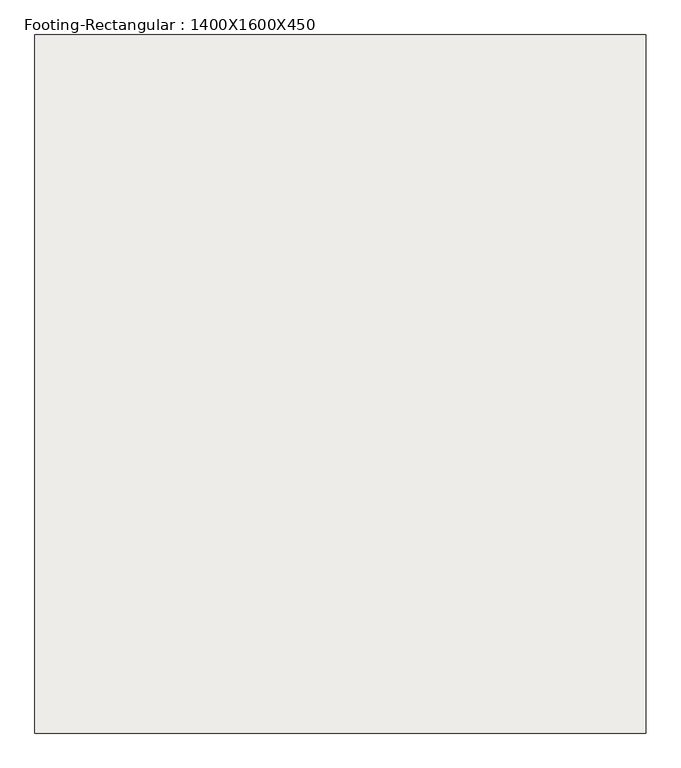
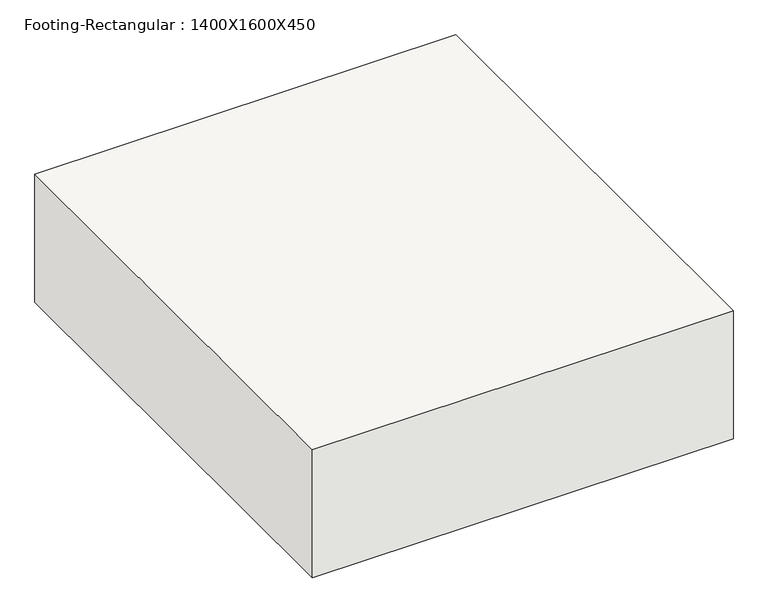
"""IFC4 building model written with IfcOpenShell, lengths in millimetres: slab geometry, Footing-Rectangular : 1400X1600X450."""

from ifc_helpers import new_model, si_unit, frame, origin, place, context, project, spatial, polyline, outline, extrude, source, transform, mapped, element, save


def footing_rectangular_1400x1600x450_119851bf(model_context):
    return source(origin(), model_context, "Body", "SweptSolid", [
        extrude(outline(polyline([(700.0, 800.0), (700.0, -800.0), (-700.0, -800.0), (-700.0, 800.0), (700.0, 800.0)])), frame((0.0, 0.0, -450.0), z_axis=(0.0, 0.0, 1.0), x_axis=(1.0, 0.0, 0.0)), (0.0, 0.0, 1.0), 450.0),
    ])


if __name__ == "__main__":
    model = new_model("IFC4")
    model_context = context("Model", 3, world=origin())
    ifc_project = project(units=[si_unit("LENGTHUNIT", "METRE", prefix="MILLI")], contexts=[model_context])
    site = spatial("IfcSite", under=ifc_project)
    building = spatial("IfcBuilding", under=site)
    placement = place(None, origin())
    footing_rectangular_1400x1600x450_shape = footing_rectangular_1400x1600x450_119851bf(model_context)
    element("IfcSlab", 1, ObjectType="Footing-Rectangular : 1400X1600X450", at=placement, inside=building, context=model_context, shape_type="MappedRepresentation", body=[
        mapped(footing_rectangular_1400x1600x450_shape, transform((0.0, 0.0, 0.0), x_axis=(1.0, 0.0, 0.0), y_axis=(0.0, 1.0, 0.0), z_axis=(0.0, 0.0, 1.0))),
    ])
    save(model, "model.ifc")

# Revit data of these elements
# Type "Footing-Rectangular : 1400X1600X450"
#   Width = 4' - 7.11811"
#   Length = 5' - 2.99213"
#   Foundation Thickness = 1' - 5.71654"
#   Structural Material [instance default] = Concrete - Cast-in-Place Concrete
#   Assembly Code = ""
# Element 1 (IfcSlab, "Footing-Rectangular : 1400X1600X450")
#   Materials on its faces: "Concrete - Cast-in-Place Concrete"
# Materials
#   "Concrete - Cast-in-Place Concrete": class "Concrete", colour RGB 192 192 192, transparency 0, Cost = 0
